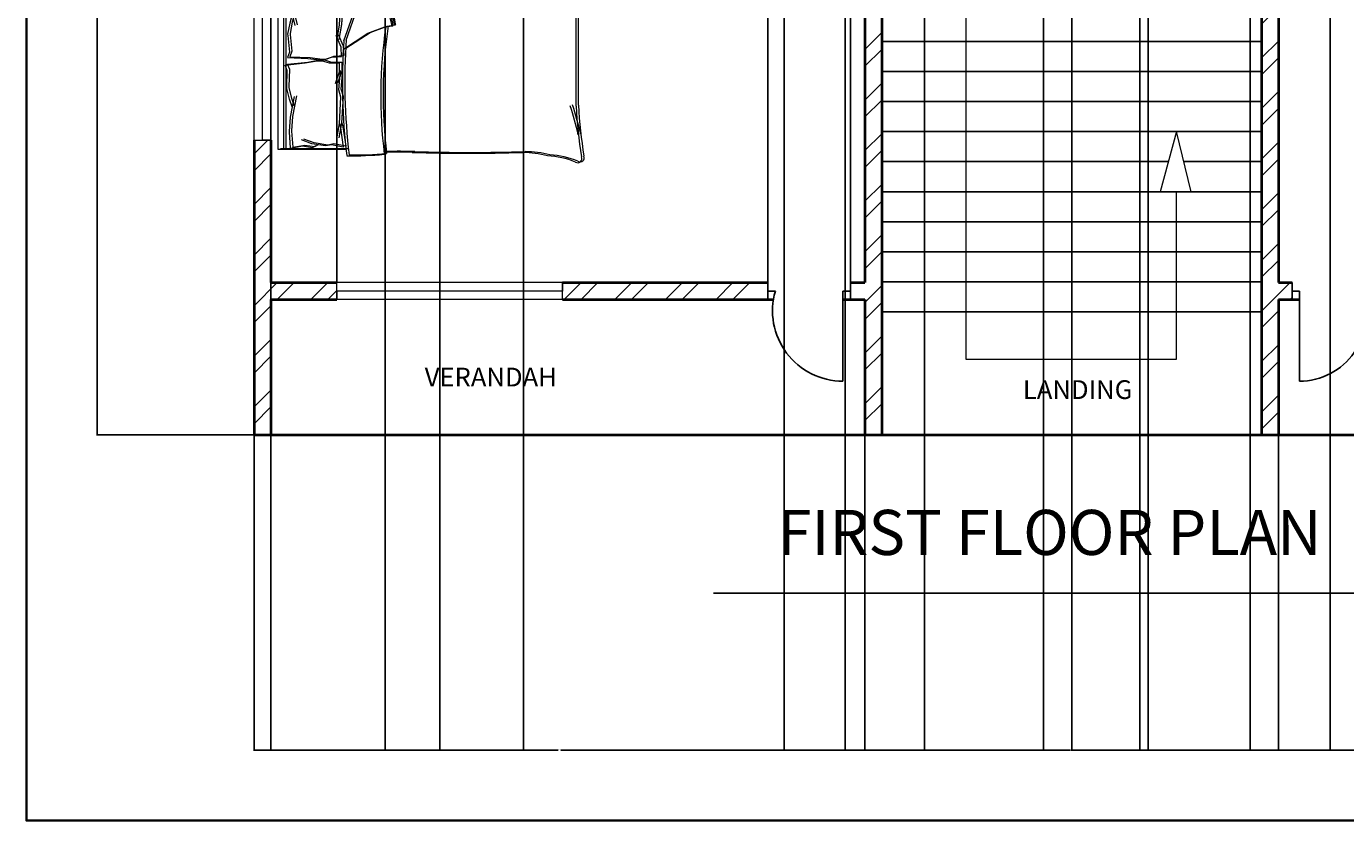
# Model space of a CAD drawing. Units: inches. Extents: x 2063 to 2617, y 1299 to 2210.
# Tile 1 of 22: x 2063 to 2414, y 1299 to 1510. Entities that reach past the tile are written whole.
import ezdxf

# ---------------------------------------------------------------- set-up
doc = ezdxf.new("R2010")
doc.units = ezdxf.units.IN
for name, color, linetype, lineweight in [('A-ANNO-DIMS', 2, 'Continuous', 18), ('A-ANNO-SYMB', 171, 'Continuous', 18), ('A-ANNO-TEXT', 7, 'Continuous', 25), ('A-ANNO-TTLB', 7, 'Continuous', 35), ('A-AREA-IDEN', 7, 'Continuous', 18), ('A-DOOR', 11, 'Continuous', 25), ('A-FLOR-STRS', 171, 'Continuous', 25), ('A-FURN', 8, 'Continuous', 18), ('A-GLAZ', 123, 'Continuous', 18), ('A-WALL', 7, 'Continuous', 40)]:
    doc.layers.add(name, color=color, linetype=linetype, lineweight=lineweight)
doc.layers.add('A-WALL-PATT', color=215, linetype='Continuous', lineweight=13, true_color=0xa953a0)
doc.styles.get("Standard").update_dxf_attribs({"font": 'arial.ttf'})
doc.dimstyles.get("Standard").update_dxf_attribs({"dimtxt": 0.18, "dimasz": 0.18, "dimexe": 0.18, "dimexo": 0.0625, "dimgap": 0.09, "dimtad": 0, "dimtih": 1, "dimtoh": 1, "dimdec": 4, "dimzin": 0, "dimdsep": 46, "dimtxsty": 'Standard', "dimcen": 0.09, "dimadec": 0, "dimazin": 0, "dimtfac": 1, "dimtdec": 4, "dimtofl": 0, "dimtmove": 0, "dimatfit": 3, "dimfxl": 1, "dimtolj": 1, "dimtzin": 0, "dimarcsym": 0})

# ---------------------------------------------------------------- blocks, each defined once
blk = doc.blocks.new('BED-DOUBLE')
for p, q in [((3.48, 63.33), (3.48, 81.44)), ((3.48, 63.33), (3.48, 81.44)), ((3.48, 81.44), (51.49, 81.44)), ((3.7, 62.69), (3.7, 80.8)), ((3.7, 62.69), (3.7, 80.8)), ((51.27, 81.44), (51.27, 54.83)), ((51.27, 81.44), (51.27, 54.83)), ((51.49, 81.44), (51.49, 80.8)), ((51.49, 80.8), (51.49, 54.19)), ((51.49, 80.8), (51.49, 54.19)), ((3.48, 79.91), (51.27, 79.91)), ((3.48, 79.91), (51.27, 79.91)), ((3.7, 79.27), (51.49, 79.27)), ((3.7, 79.27), (51.49, 79.27)), ((3.89, 78.13), (4.47, 74.95)), ((3.9, 78.11), (8.18, 78.43)), ((3.9, 78.11), (8.18, 78.43)), ((3.9, 78.13), (4.47, 74.95)), ((4.12, 77.49), (4.7, 74.31)), ((4.12, 77.49), (4.7, 74.31)), ((4.13, 77.47), (8.41, 77.8)), ((4.13, 77.47), (8.41, 77.8)), ((8.18, 78.43), (8.29, 78.42)), ((8.18, 78.43), (8.29, 78.42)), ((8.29, 78.42), (12.11, 78.13)), ((8.29, 78.42), (12.11, 78.13)), ((8.41, 77.8), (8.51, 77.78)), ((8.41, 77.8), (8.51, 77.78)), ((8.51, 77.78), (12.34, 77.49)), ((8.51, 77.78), (12.34, 77.49)), ((12.11, 78.13), (17.6, 77.12)), ((12.11, 78.13), (17.6, 77.12)), ((12.34, 77.49), (17.83, 76.48)), ((12.34, 77.49), (17.83, 76.48)), ((14.86, 77.69), (16.88, 78.42)), ((14.86, 77.69), (16.88, 78.42)), ((15.08, 77.05), (17.11, 77.78)), ((15.08, 77.05), (17.11, 77.78)), ((16.88, 78.42), (19.77, 79.14)), ((16.88, 78.42), (19.77, 79.14)), ((17.11, 77.78), (20, 78.5)), ((17.11, 77.78), (20, 78.5)), ((19.77, 79.14), (20.09, 79.14)), ((19.77, 79.14), (20.09, 79.14)), ((20, 78.5), (20.32, 78.5)), ((20, 78.5), (20.32, 78.5)), ((20.09, 79.14), (24.54, 79)), ((20.09, 79.14), (24.54, 79)), ((20.32, 78.5), (24.77, 78.36)), ((20.32, 78.5), (24.77, 78.36)), ((24.54, 79), (25.98, 79.57)), ((24.54, 79), (25.98, 79.57)), ((24.77, 78.36), (26.21, 78.93)), ((24.77, 78.36), (26.21, 78.93)), ((25.98, 79.57), (26.56, 74.22)), ((25.98, 79.57), (26.56, 74.22)), ((26.21, 78.93), (26.79, 73.58)), ((26.21, 78.93), (26.79, 73.58)), ((27.98, 78.95), (27.73, 73.58)), ((27.98, 78.95), (27.73, 73.58)), ((28.21, 78.31), (27.96, 72.94)), ((28.21, 78.31), (27.96, 72.94)), ((29.46, 78.46), (27.98, 78.95)), ((29.46, 78.46), (27.98, 78.95)), ((29.68, 77.83), (28.21, 78.31)), ((29.68, 77.83), (28.21, 78.31)), ((33.88, 78.89), (29.46, 78.46)), ((33.88, 78.89), (29.46, 78.46)), ((34.11, 78.25), (29.68, 77.83)), ((34.11, 78.25), (29.68, 77.83)), ((34.21, 78.91), (33.88, 78.89)), ((34.2, 78.91), (33.88, 78.89)), ((34.43, 78.27), (34.11, 78.25)), ((34.43, 78.27), (34.11, 78.25)), ((37.14, 78.37), (34.2, 78.91)), ((37.14, 78.37), (34.21, 78.91)), ((37.36, 77.73), (34.43, 78.27)), ((37.36, 77.73), (34.43, 78.27)), ((41.91, 78.37), (36.5, 77.02)), ((41.91, 78.37), (36.5, 77.02)), ((42.14, 77.73), (36.72, 76.38)), ((42.14, 77.73), (36.72, 76.38)), ((39.2, 77.77), (37.14, 78.37)), ((39.2, 77.77), (37.14, 78.37)), ((39.43, 77.13), (37.36, 77.73)), ((39.43, 77.13), (37.36, 77.73)), ((45.71, 78.9), (41.91, 78.37)), ((45.71, 78.9), (41.91, 78.37)), ((45.94, 78.26), (42.14, 77.73)), ((45.94, 78.26), (42.14, 77.73)), ((50.11, 78.89), (44.71, 78.98)), ((44.71, 78.98), (45.71, 78.9)), ((50.11, 78.89), (44.71, 78.98)), ((44.71, 78.98), (45.71, 78.9)), ((50.34, 78.25), (44.94, 78.34)), ((44.94, 78.34), (45.94, 78.26)), ((50.34, 78.25), (44.94, 78.34)), ((44.94, 78.34), (45.94, 78.26)), ((50.11, 78.89), (49.73, 75.68)), ((50.11, 78.89), (49.73, 75.68)), ((50.34, 78.25), (49.96, 75.04)), ((50.34, 78.25), (49.96, 75.04)), ((4.47, 74.95), (4.04, 72.34)), ((4.47, 74.95), (4.04, 72.34)), ((4.7, 74.31), (4.27, 71.7)), ((4.7, 74.31), (4.27, 71.7)), ((5.05, 72.49), (6.06, 75.24)), ((5.05, 72.49), (6.06, 75.24)), ((5.28, 71.85), (6.29, 74.6)), ((5.28, 71.85), (6.29, 74.6)), ((26.56, 74.22), (27.14, 71.04)), ((26.56, 74.22), (27.14, 71.04)), ((49.31, 73.19), (48.13, 75.87)), ((49.31, 73.19), (48.13, 75.87)), ((49.54, 72.55), (48.36, 75.23)), ((49.54, 72.55), (48.36, 75.23)), ((49.73, 75.68), (50.33, 73.11)), ((49.73, 75.68), (50.33, 73.11)), ((49.96, 75.04), (50.56, 72.47)), ((49.96, 75.04), (50.56, 72.47)), ((4.04, 72.34), (4.62, 71.33)), ((4.04, 72.34), (4.62, 71.33)), ((4.27, 71.7), (4.85, 70.69)), ((4.27, 71.7), (4.85, 70.69)), ((4.47, 68.87), (5.05, 72.49)), ((4.47, 68.87), (5.05, 72.49)), ((4.7, 68.23), (5.28, 71.85)), ((4.7, 68.23), (5.28, 71.85)), ((26.79, 73.58), (27.37, 70.4)), ((26.79, 73.58), (27.37, 70.4)), ((27.14, 71.04), (27.14, 69.74)), ((27.14, 71.04), (27.14, 69.74)), ((27.73, 73.58), (27.36, 70.37)), ((27.73, 73.58), (27.36, 70.37)), ((27.36, 70.37), (27.44, 69.07)), ((27.36, 70.37), (27.44, 69.07)), ((27.37, 70.4), (27.37, 69.1)), ((27.37, 70.4), (27.37, 69.1)), ((27.96, 72.94), (27.58, 69.73)), ((27.96, 72.94), (27.58, 69.73)), ((50.11, 69.61), (49.31, 73.19)), ((50.11, 69.61), (49.31, 73.19)), ((50.34, 68.98), (49.54, 72.55)), ((50.34, 68.98), (49.54, 72.55)), ((50.33, 73.11), (49.81, 72.06)), ((50.33, 73.11), (49.82, 72.06)), ((50.56, 72.47), (50.04, 71.42)), ((50.56, 72.47), (50.04, 71.42)), ((4.18, 64.1), (4.76, 67.28)), ((4.18, 64.1), (4.76, 67.28)), ((4.76, 67.28), (4.47, 68.87)), ((4.76, 67.28), (4.47, 68.87)), ((4.99, 66.64), (4.7, 68.23)), ((4.99, 66.64), (4.7, 68.23)), ((27.14, 69.74), (26.56, 67.86)), ((27.14, 69.74), (26.56, 67.86)), ((26.56, 67.86), (26.56, 65.18)), ((26.56, 67.86), (26.56, 65.18)), ((27.37, 69.1), (26.79, 67.22)), ((27.37, 69.1), (26.79, 67.22)), ((26.79, 67.22), (26.79, 64.54)), ((26.79, 67.22), (26.79, 64.54)), ((27.44, 69.07), (28.13, 67.23)), ((27.44, 69.07), (28.13, 67.23)), ((27.58, 69.73), (27.66, 68.43)), ((27.58, 69.73), (27.66, 68.43)), ((27.66, 68.43), (28.36, 66.59)), ((27.66, 68.43), (28.36, 66.59)), ((28.13, 67.23), (28.3, 64.55)), ((28.13, 67.23), (28.3, 64.55)), ((49.92, 68.01), (50.11, 69.61)), ((49.92, 68.01), (50.11, 69.61)), ((50.7, 64.87), (49.92, 68.01)), ((50.7, 64.87), (49.92, 68.01)), ((50.15, 67.37), (50.34, 68.98)), ((50.15, 67.37), (50.34, 68.98)), ((50.93, 64.23), (50.15, 67.37)), ((50.93, 64.23), (50.15, 67.37)), ((9.28, 64.83), (4.18, 64.1)), ((9.28, 64.83), (4.18, 64.1)), ((4.41, 63.46), (4.99, 66.64)), ((4.41, 63.46), (4.99, 66.64)), ((9.51, 64.19), (4.41, 63.46)), ((9.51, 64.19), (4.41, 63.46)), ((6.38, 65.82), (10.41, 65.15)), ((6.38, 65.82), (10.41, 65.15)), ((6.61, 65.18), (10.64, 64.51)), ((6.61, 65.18), (10.64, 64.51)), ((10.41, 65.15), (9.28, 64.83)), ((10.41, 65.15), (9.28, 64.83)), ((10.64, 64.51), (9.51, 64.19)), ((10.64, 64.51), (9.51, 64.19)), ((10.41, 65.15), (17.42, 64.72)), ((10.41, 65.15), (17.42, 64.72)), ((10.64, 64.51), (17.65, 64.08)), ((10.64, 64.51), (17.65, 64.08)), ((17.42, 64.72), (19.38, 65.27)), ((17.42, 64.72), (19.38, 65.27)), ((17.65, 64.08), (19.61, 64.64)), ((17.65, 64.08), (19.61, 64.64)), ((19.38, 65.27), (24.52, 64.87)), ((19.38, 65.27), (24.52, 64.87)), ((19.61, 64.64), (24.74, 64.23)), ((19.61, 64.64), (24.74, 64.23)), ((24.1, 65.18), (20.96, 66.27)), ((24.1, 65.18), (20.96, 66.27)), ((24.33, 64.54), (21.19, 65.63)), ((24.33, 64.54), (21.19, 65.63)), ((26.56, 65.18), (24.1, 65.18)), ((26.56, 65.18), (24.1, 65.18)), ((26.79, 64.54), (24.33, 64.54)), ((26.79, 64.54), (24.33, 64.54)), ((28.3, 64.55), (30.75, 64.7)), ((28.3, 64.55), (30.75, 64.7)), ((28.36, 66.59), (28.53, 63.91)), ((28.36, 66.59), (28.53, 63.91)), ((28.53, 63.91), (30.98, 64.06)), ((28.53, 63.91), (30.98, 64.06)), ((30.26, 64.06), (34.45, 57.57)), ((30.26, 64.06), (34.45, 57.57)), ((30.49, 63.42), (34.68, 56.93)), ((30.49, 63.42), (34.68, 56.93)), ((30.75, 64.7), (33.82, 65.99)), ((30.75, 64.7), (33.82, 65.99)), ((30.98, 64.06), (34.05, 65.35)), ((30.98, 64.06), (34.05, 65.35)), ((40.64, 61.13), (32.31, 64.06)), ((40.64, 61.13), (32.31, 64.06)), ((40.87, 60.49), (32.53, 63.42)), ((40.87, 60.49), (32.54, 63.42)), ((32.56, 65.82), (36.6, 65.15)), ((32.56, 65.82), (36.6, 65.15)), ((32.79, 65.18), (36.83, 64.51)), ((32.79, 65.18), (36.82, 64.51)), ((36.6, 65.15), (43.61, 64.72)), ((36.6, 65.15), (43.61, 64.72)), ((36.82, 64.51), (43.83, 64.08)), ((36.83, 64.51), (43.84, 64.08)), ((43.61, 64.72), (45.57, 65.27)), ((43.61, 64.72), (45.57, 65.27)), ((43.83, 64.08), (45.8, 64.64)), ((43.84, 64.08), (45.8, 64.64)), ((45.57, 65.27), (50.7, 64.87)), ((45.57, 65.27), (50.7, 64.87)), ((45.8, 64.64), (50.93, 64.23)), ((45.8, 64.64), (50.93, 64.23)), ((46.22, 59.11), (40.64, 61.13)), ((46.22, 59.11), (40.64, 61.13)), ((46.45, 58.48), (40.87, 60.49)), ((46.45, 58.48), (40.87, 60.49)), ((34.45, 57.57), (36.15, 53.08)), ((34.45, 57.57), (36.15, 53.08)), ((34.68, 56.93), (36.38, 52.44)), ((34.68, 56.93), (36.38, 52.44)), ((49.16, 56.95), (46.22, 59.11)), ((49.16, 56.95), (46.22, 59.11)), ((49.39, 56.31), (46.45, 58.48)), ((49.39, 56.31), (46.45, 58.48)), ((52.87, 53.7), (49.16, 56.95)), ((52.87, 53.7), (49.16, 56.95)), ((53.1, 53.06), (49.39, 56.31)), ((53.1, 53.06), (49.39, 56.31)), ((36.15, 53.08), (36.46, 51.07)), ((36.15, 53.08), (36.46, 51.07)), ((40.95, 52.61), (44.36, 53.08)), ((40.95, 52.61), (44.36, 53.08)), ((44.36, 53.08), (48.23, 53.39)), ((44.36, 53.08), (48.23, 53.39)), ((44.59, 52.44), (48.46, 52.75)), ((44.59, 52.44), (48.46, 52.75)), ((48.23, 53.39), (51.33, 53.08)), ((48.23, 53.39), (51.33, 53.08)), ((48.46, 52.75), (51.56, 52.44)), ((48.46, 52.75), (51.56, 52.44)), ((51.33, 53.08), (52.87, 53.7)), ((51.33, 53.08), (52.87, 53.7)), ((51.56, 52.44), (53.1, 53.06)), ((51.56, 52.44), (53.1, 53.06)), ((52.95, 51.95), (52.87, 53.7, 3.87)), ((52.95, 51.95), (52.87, 53.7, 3.87)), ((53.18, 51.31), (53.1, 53.06, 3.87)), ((53.18, 51.31), (53.1, 53.06, 3.87)), ((36.38, 52.44), (36.69, 50.43)), ((36.38, 52.44), (36.69, 50.43)), ((36.46, 51.07), (38.94, 51.69)), ((36.46, 51.07), (38.94, 51.69)), ((36.69, 50.43), (39.17, 51.05)), ((36.69, 50.43), (39.17, 51.05)), ((38.94, 51.69), (40.95, 52.61)), ((38.94, 51.69), (40.95, 52.61)), ((39.17, 51.05), (41.18, 51.97)), ((39.17, 51.05), (41.18, 51.97)), ((41.18, 51.97), (44.59, 52.44)), ((41.18, 51.97), (44.59, 52.44)), ((15.06, 2.2), (39.68, 2.2)), ((15.06, 2.2), (39.68, 2.2)), ((15.29, 1.56), (39.91, 1.56)), ((15.29, 1.56), (39.91, 1.56))]:
    blk.add_line(p, q)
for centre, radius, start, end in [((85.16, 61.35), 83.31, 178.7218, 185.604), ((85.16, 61.35), 83.31, 178.7218, 185.604), ((21.36, -100.61), 164.97, 86.0865, 96.7821), ((21.36, -100.61), 164.97, 86.0865, 96.7821), ((21.59, -101.25), 164.97, 86.0865, 96.7821), ((21.59, -101.25), 164.97, 86.0865, 96.7821), ((85.39, 60.71), 83.31, 178.7218, 185.604), ((85.39, 60.71), 83.31, 178.7218, 185.604), ((17.76, -74.87), 129.02, 81.7845, 96.9006), ((17.76, -74.87), 129.02, 81.7845, 96.9006), ((17.98, -75.51), 129.02, 81.7845, 96.9006), ((17.98, -75.51), 129.02, 81.7845, 96.9006), ((-167.31, 50.27), 170.11, 358.4762, 1.0082), ((-167.31, 50.27), 170.11, 358.4762, 1.0082), ((-167.08, 49.63), 170.11, 358.4762, 1.0082), ((-167.08, 49.63), 170.11, 358.4762, 1.0082), ((36.64, 51), 0.185, 160.2464, 271.1377), ((36.64, 51), 0.185, 160.2464, 271.1377), ((31.15, 79.96), 29.65, 280.6617, 289.8806), ((31.15, 79.96), 29.65, 280.6617, 289.8806), ((36.87, 50.36), 0.185, 160.2464, 271.1377), ((36.86, 50.36), 0.185, 160.2464, 271.1377), ((31.38, 79.32), 29.65, 280.6617, 289.8806), ((31.38, 79.32), 29.65, 280.6617, 289.8806), ((43.74, 46.38), 6.22, 78.6608, 113.7384), ((43.74, 46.38), 6.22, 78.6608, 113.7384), ((43.97, 45.74), 6.22, 78.6608, 113.7384), ((43.97, 45.74), 6.22, 78.6608, 113.7384), ((51.33, 88.1), 36.18, 259.8763, 272.5657), ((51.33, 88.1), 36.18, 259.8763, 272.5657), ((51.56, 87.46), 36.18, 259.8763, 272.5657), ((51.56, 87.46), 36.18, 259.8763, 272.5657), ((182.27, 45.13), 129.5, 176.9791, 183.8365), ((182.27, 45.13), 129.5, 176.9791, 183.8365), ((182.49, 44.49), 129.5, 176.9791, 183.8365), ((182.49, 44.49), 129.5, 176.9791, 183.8365), ((484.82, 30.83), 482.31, 178.2277, 181.7185), ((484.82, 30.83), 482.31, 178.2277, 181.7185), ((485.05, 30.19), 482.31, 178.2277, 181.7185), ((485.05, 30.19), 482.31, 178.2277, 181.7185), ((-4508.74, 13.62), 4561.86, 0.00217, 0.28689), ((-4508.74, 13.62), 4561.86, 0.00217, 0.28689), ((-4508.51, 12.98), 4561.86, 0.00217, 0.28689), ((-4508.51, 12.98), 4561.86, 0.00217, 0.28689), ((-26.9, 16.93), 29.63, 346.0648, 358.9113), ((-26.9, 16.93), 29.63, 346.0648, 358.9113), ((-26.67, 16.29), 29.63, 346.0648, 358.9113), ((-26.67, 16.29), 29.63, 346.0648, 358.9113), ((76.16, 12.78), 23.07, 177.4714, 206.4681), ((76.16, 12.78), 23.07, 177.4714, 206.4681), ((76.39, 12.14), 23.07, 177.4714, 206.4681), ((76.39, 12.14), 23.07, 177.4714, 206.4681), ((-21.66, 11.17), 23.56, 337.9751, 356.652), ((-21.66, 11.17), 23.56, 337.9751, 356.652), ((-21.43, 10.53), 23.56, 337.9751, 356.652), ((-21.43, 10.53), 23.56, 337.9751, 356.652), ((-17.22, 105.16), 106.46, 283.3832, 287.7053), ((-17.22, 105.16), 106.46, 283.3832, 287.7053), ((1.09, 1.73), 1.09, 146.1736, 293.4781), ((1.09, 1.73), 1.09, 146.1736, 293.4781), ((1.32, 1.09), 1.09, 146.1736, 293.4781), ((1.32, 1.09), 1.09, 146.1736, 293.4781), ((21.43, -119.39), 121.76, 92.9958, 99.4091), ((21.43, -119.39), 121.76, 92.9958, 99.4091), ((21.66, -120.03), 121.76, 92.9958, 99.4091), ((21.66, -120.03), 121.76, 92.9958, 99.4091), ((-16.99, 104.52), 106.46, 283.3832, 287.7053), ((-16.99, 104.52), 106.46, 283.3832, 287.7053), ((41.15, -130.83), 133.04, 84.4998, 90.6351), ((41.15, -130.83), 133.04, 84.4998, 90.6351), ((41.38, -131.47), 133.04, 84.4998, 90.6351), ((41.38, -131.47), 133.04, 84.4998, 90.6351), ((54.41, 2.57), 1.1, 242.6588, 356.02), ((54.41, 2.57), 1.1, 242.6588, 356.02), ((54.64, 1.93), 1.1, 242.6588, 356.02), ((54.64, 1.93), 1.1, 242.6588, 356.02)]:
    blk.add_arc(centre, radius, start, end)
blk = doc.blocks.new('WIN-60IN')
for p, q in [((0, 60), (4.5, 60)), ((0, 60), (0, 0)), ((4.5, 60), (2.25, 60)), ((2.25, 60), (2.25, 0)), ((4.5, 60), (4.5, 0)), ((2.25, 0), (0, 0)), ((0, 0), (4.5, 0))]:
    blk.add_line(p, q)
blk = doc.blocks.new('*D32')
at = {"layer": 'A-ANNO-DIMS', "color": 0, "lineweight": -2, "transparency": 16777216}
for p, q in [((2123.08, 2128.81), (2081.21, 2128.81)), ((2081.39, 2128.63), (2081.39, 1765.49)), ((2081.39, 1401.99), (2081.39, 1765.13)), ((2123.08, 1401.81), (2081.21, 1401.81))]:
    blk.add_line(p, q, dxfattribs=at)
at = {"layer": 'A-ANNO-DIMS', "color": 0, "transparency": 16777216}
for points in [[(2081.36, 2128.63), (2081.42, 2128.63), (2081.39, 2128.81)], [(2081.36, 1401.99), (2081.42, 1401.99), (2081.39, 1401.81)]]:
    blk.add_solid(points, dxfattribs=at)
at = {"layer": 'Defpoints', "color": 0, "transparency": 16777216}
for p in [(2081.39, 2128.81), (2123.14, 2128.81), (2123.14, 1401.81)]:
    blk.add_point(p, dxfattribs=at)
at = {"layer": 'A-ANNO-DIMS', "color": 0, "transparency": 16777216, "insert": (2081.39, 1765.31), "char_height": 0.18, "attachment_point": 5}
blk.add_mtext('\\A1;727', dxfattribs=at)
blk = doc.blocks.new('*D33')
at = {"layer": 'A-ANNO-DIMS', "color": 0, "lineweight": -2, "transparency": 16777216}
for p, q in [((2123.14, 1401.75), (2123.14, 1317.7)), ((2285.64, 1401.75), (2285.64, 1317.7)), ((2123.32, 1317.88), (2204.01, 1317.88)), ((2285.46, 1317.88), (2204.78, 1317.88))]:
    blk.add_line(p, q, dxfattribs=at)
at = {"layer": 'A-ANNO-DIMS', "color": 0, "transparency": 16777216}
for points in [[(2123.32, 1317.91), (2123.32, 1317.85), (2123.14, 1317.88)], [(2285.46, 1317.91), (2285.46, 1317.85), (2285.64, 1317.88)]]:
    blk.add_solid(points, dxfattribs=at)
at = {"layer": 'Defpoints', "color": 0, "transparency": 16777216}
for p in [(2123.14, 1401.81), (2285.64, 1401.81), (2285.64, 1317.88)]:
    blk.add_point(p, dxfattribs=at)
at = {"layer": 'A-ANNO-DIMS', "color": 0, "transparency": 16777216, "insert": (2204.39, 1317.88), "char_height": 0.18, "attachment_point": 5}
blk.add_mtext('\\A1;162.5', dxfattribs=at)
blk = doc.blocks.new('*D34')
at = {"layer": 'A-ANNO-DIMS', "color": 0, "lineweight": -2, "transparency": 16777216}
for p, q in [((2285.64, 1401.75), (2285.64, 1317.7)), ((2395.64, 1401.75), (2395.64, 1317.7)), ((2285.82, 1317.88), (2340.36, 1317.88)), ((2395.46, 1317.88), (2340.92, 1317.88))]:
    blk.add_line(p, q, dxfattribs=at)
at = {"layer": 'A-ANNO-DIMS', "color": 0, "transparency": 16777216}
for points in [[(2285.82, 1317.91), (2285.82, 1317.85), (2285.64, 1317.88)], [(2395.46, 1317.91), (2395.46, 1317.85), (2395.64, 1317.88)]]:
    blk.add_solid(points, dxfattribs=at)
at = {"layer": 'Defpoints', "color": 0, "transparency": 16777216}
for p in [(2285.64, 1401.81), (2395.64, 1401.81), (2395.64, 1317.88)]:
    blk.add_point(p, dxfattribs=at)
at = {"layer": 'A-ANNO-DIMS', "color": 0, "transparency": 16777216, "insert": (2340.64, 1317.88), "char_height": 0.18, "attachment_point": 5}
blk.add_mtext('\\A1;110', dxfattribs=at)
blk = doc.blocks.new('*D35')
at = {"layer": 'A-ANNO-DIMS', "color": 0, "lineweight": -2, "transparency": 16777216}
for p, q in [((2395.64, 1401.75), (2395.64, 1317.7)), ((2553.64, 1401.75), (2553.64, 1317.7)), ((2395.82, 1317.88), (2474.36, 1317.88)), ((2553.46, 1317.88), (2474.92, 1317.88))]:
    blk.add_line(p, q, dxfattribs=at)
at = {"layer": 'A-ANNO-DIMS', "color": 0, "transparency": 16777216}
for points in [[(2395.82, 1317.91), (2395.82, 1317.85), (2395.64, 1317.88)], [(2553.46, 1317.91), (2553.46, 1317.85), (2553.64, 1317.88)]]:
    blk.add_solid(points, dxfattribs=at)
at = {"layer": 'Defpoints', "color": 0, "transparency": 16777216}
for p in [(2395.64, 1401.81), (2553.64, 1401.81), (2553.64, 1317.88)]:
    blk.add_point(p, dxfattribs=at)
at = {"layer": 'A-ANNO-DIMS', "color": 0, "transparency": 16777216, "insert": (2474.64, 1317.88), "char_height": 0.18, "attachment_point": 5}
blk.add_mtext('\\A1;158', dxfattribs=at)
blk = doc.blocks.new('*D49')
at = {"layer": 'A-ANNO-DIMS', "color": 0, "lineweight": -2, "transparency": 16777216}
for p, q in [((2127.64, 2124.25), (2127.64, 1317.7)), ((2158.04, 2124.25), (2158.04, 1317.7)), ((2127.82, 1317.88), (2142.38, 1317.88)), ((2157.86, 1317.88), (2143.31, 1317.88))]:
    blk.add_line(p, q, dxfattribs=at)
at = {"layer": 'A-ANNO-DIMS', "color": 0, "transparency": 16777216}
for points in [[(2127.82, 1317.91), (2127.82, 1317.85), (2127.64, 1317.88)], [(2157.86, 1317.91), (2157.86, 1317.85), (2158.04, 1317.88)]]:
    blk.add_solid(points, dxfattribs=at)
at = {"layer": 'Defpoints', "color": 0, "transparency": 16777216}
for p in [(2127.64, 2124.31), (2158.04, 2124.31), (2158.04, 1317.88)]:
    blk.add_point(p, dxfattribs=at)
at = {"layer": 'A-ANNO-DIMS', "color": 0, "transparency": 16777216, "insert": (2142.84, 1317.88), "char_height": 0.18, "attachment_point": 5}
blk.add_mtext('\\A1;30.396', dxfattribs=at)
blk = doc.blocks.new('*D50')
at = {"layer": 'A-ANNO-DIMS', "color": 0, "lineweight": -2, "transparency": 16777216}
for p, q in [((2264.14, 2124.25), (2264.14, 1317.7)), ((2280.35, 2124.25), (2280.35, 1317.7)), ((2264.32, 1317.88), (2271.79, 1317.88)), ((2280.17, 1317.88), (2272.7, 1317.88))]:
    blk.add_line(p, q, dxfattribs=at)
at = {"layer": 'A-ANNO-DIMS', "color": 0, "transparency": 16777216}
for points in [[(2264.32, 1317.91), (2264.32, 1317.85), (2264.14, 1317.88)], [(2280.17, 1317.91), (2280.17, 1317.85), (2280.35, 1317.88)]]:
    blk.add_solid(points, dxfattribs=at)
at = {"layer": 'Defpoints', "color": 0, "transparency": 16777216}
for p in [(2264.14, 2124.31), (2280.35, 2124.31), (2280.35, 1317.88)]:
    blk.add_point(p, dxfattribs=at)
at = {"layer": 'A-ANNO-DIMS', "color": 0, "transparency": 16777216, "insert": (2272.25, 1317.88), "char_height": 0.18, "attachment_point": 5}
blk.add_mtext('\\A1;16.204', dxfattribs=at)
blk = doc.blocks.new('*D51')
at = {"layer": 'A-ANNO-DIMS', "color": 0, "lineweight": -2, "transparency": 16777216}
for p, q in [((2340.64, 2124.25), (2340.64, 1317.7)), ((2358.75, 2124.25), (2358.75, 1317.7)), ((2340.82, 1317.88), (2349.24, 1317.88)), ((2358.57, 1317.88), (2350.15, 1317.88))]:
    blk.add_line(p, q, dxfattribs=at)
at = {"layer": 'A-ANNO-DIMS', "color": 0, "transparency": 16777216}
for points in [[(2340.82, 1317.91), (2340.82, 1317.85), (2340.64, 1317.88)], [(2358.57, 1317.91), (2358.57, 1317.85), (2358.75, 1317.88)]]:
    blk.add_solid(points, dxfattribs=at)
at = {"layer": 'Defpoints', "color": 0, "transparency": 16777216}
for p in [(2340.64, 2124.31), (2358.75, 2124.31), (2358.75, 1317.88)]:
    blk.add_point(p, dxfattribs=at)
at = {"layer": 'A-ANNO-DIMS', "color": 0, "transparency": 16777216, "insert": (2349.7, 1317.88), "char_height": 0.18, "attachment_point": 5}
blk.add_mtext('\\A1;18.106', dxfattribs=at)
blk = doc.blocks.new('*D54')
at = {"layer": 'A-ANNO-DIMS', "color": 0, "lineweight": -2, "transparency": 16777216}
for p, q in [((2340.64, 2124.25), (2340.64, 1317.7)), ((2360.96, 2104.46), (2360.96, 1317.7)), ((2340.82, 1317.88), (2350.34, 1317.88)), ((2360.78, 1317.88), (2351.27, 1317.88))]:
    blk.add_line(p, q, dxfattribs=at)
at = {"layer": 'A-ANNO-DIMS', "color": 0, "transparency": 16777216}
for points in [[(2340.82, 1317.91), (2340.82, 1317.85), (2340.64, 1317.88)], [(2360.78, 1317.91), (2360.78, 1317.85), (2360.96, 1317.88)]]:
    blk.add_solid(points, dxfattribs=at)
at = {"layer": 'Defpoints', "color": 0, "transparency": 16777216}
for p in [(2340.64, 2124.31), (2360.96, 2104.52), (2360.96, 1317.88)]:
    blk.add_point(p, dxfattribs=at)
at = {"layer": 'A-ANNO-DIMS', "color": 0, "transparency": 16777216, "insert": (2350.8, 1317.88), "char_height": 0.18, "attachment_point": 5}
blk.add_mtext('\\A1;20.317', dxfattribs=at)
blk = doc.blocks.new('*D55')
at = {"layer": 'A-ANNO-DIMS', "color": 0, "lineweight": -2, "transparency": 16777216}
for p, q in [((2388.15, 1975.75), (2388.15, 1317.7)), ((2409.37, 1975.75), (2409.37, 1317.7)), ((2388.33, 1317.88), (2398.3, 1317.88)), ((2409.19, 1317.88), (2399.23, 1317.88))]:
    blk.add_line(p, q, dxfattribs=at)
at = {"layer": 'A-ANNO-DIMS', "color": 0, "transparency": 16777216}
for points in [[(2388.33, 1317.91), (2388.33, 1317.85), (2388.15, 1317.88)], [(2409.19, 1317.91), (2409.19, 1317.85), (2409.37, 1317.88)]]:
    blk.add_solid(points, dxfattribs=at)
at = {"layer": 'Defpoints', "color": 0, "transparency": 16777216}
for p in [(2388.15, 1975.81), (2409.37, 1975.81), (2409.37, 1317.88)]:
    blk.add_point(p, dxfattribs=at)
at = {"layer": 'A-ANNO-DIMS', "color": 0, "transparency": 16777216, "insert": (2398.76, 1317.88), "char_height": 0.18, "attachment_point": 5}
blk.add_mtext('\\A1;21.225', dxfattribs=at)
blk = doc.blocks.new('*D57')
at = {"layer": 'A-ANNO-DIMS', "color": 0, "lineweight": -2, "transparency": 16777216}
for p, q in [((2172.52, 1868.25), (2172.52, 1317.7)), ((2194.82, 1868.25), (2194.82, 1317.7)), ((2172.7, 1317.88), (2183.2, 1317.88)), ((2194.64, 1317.88), (2184.14, 1317.88))]:
    blk.add_line(p, q, dxfattribs=at)
at = {"layer": 'A-ANNO-DIMS', "color": 0, "transparency": 16777216}
for points in [[(2172.7, 1317.91), (2172.7, 1317.85), (2172.52, 1317.88)], [(2194.64, 1317.91), (2194.64, 1317.85), (2194.82, 1317.88)]]:
    blk.add_solid(points, dxfattribs=at)
at = {"layer": 'Defpoints', "color": 0, "transparency": 16777216}
for p in [(2172.52, 1868.31), (2194.82, 1868.31), (2194.82, 1317.88)]:
    blk.add_point(p, dxfattribs=at)
at = {"layer": 'A-ANNO-DIMS', "color": 0, "transparency": 16777216, "insert": (2183.67, 1317.88), "char_height": 0.18, "attachment_point": 5}
blk.add_mtext('\\A1;22.305', dxfattribs=at)
blk = doc.blocks.new('*D60')
at = {"layer": 'A-ANNO-DIMS', "color": 0, "lineweight": -2, "transparency": 16777216}
for p, q in [((2301.46, 1614.75), (2301.46, 1317.7)), ((2333.14, 1614.75), (2333.14, 1317.7)), ((2301.64, 1317.88), (2316.84, 1317.88)), ((2332.96, 1317.88), (2317.76, 1317.88))]:
    blk.add_line(p, q, dxfattribs=at)
at = {"layer": 'A-ANNO-DIMS', "color": 0, "transparency": 16777216}
for points in [[(2301.64, 1317.91), (2301.64, 1317.85), (2301.46, 1317.88)], [(2332.96, 1317.91), (2332.96, 1317.85), (2333.14, 1317.88)]]:
    blk.add_solid(points, dxfattribs=at)
at = {"layer": 'Defpoints', "color": 0, "transparency": 16777216}
for p in [(2301.46, 1614.81), (2333.14, 1614.81), (2333.14, 1317.88)]:
    blk.add_point(p, dxfattribs=at)
at = {"layer": 'A-ANNO-DIMS', "color": 0, "transparency": 16777216, "insert": (2317.3, 1317.88), "char_height": 0.18, "attachment_point": 5}
blk.add_mtext('\\A1;31.684', dxfattribs=at)
blk = doc.blocks.new('*D61')
at = {"layer": 'A-ANNO-DIMS', "color": 0, "lineweight": -2, "transparency": 16777216}
for p, q in [((2127.64, 1442.37), (2127.64, 2170.74)), ((2127.82, 2170.56), (2136.03, 2170.56)), ((2144.97, 2170.56), (2136.77, 2170.56)), ((2145.15, 1442.37), (2145.15, 2170.74))]:
    blk.add_line(p, q, dxfattribs=at)
at = {"layer": 'A-ANNO-DIMS', "color": 0, "transparency": 16777216}
for points in [[(2127.82, 2170.59), (2127.82, 2170.53), (2127.64, 2170.56)], [(2144.97, 2170.59), (2144.97, 2170.53), (2145.15, 2170.56)]]:
    blk.add_solid(points, dxfattribs=at)
at = {"layer": 'Defpoints', "color": 0, "transparency": 16777216}
for p in [(2145.15, 2170.56), (2127.64, 1442.31), (2145.15, 1442.31)]:
    blk.add_point(p, dxfattribs=at)
at = {"layer": 'A-ANNO-DIMS', "color": 0, "transparency": 16777216, "insert": (2136.4, 2170.56), "char_height": 0.18, "attachment_point": 5}
blk.add_mtext('\\A1;17.51', dxfattribs=at)
blk = doc.blocks.new('*D62')
at = {"layer": 'A-ANNO-DIMS', "color": 0, "lineweight": -2, "transparency": 16777216}
for p, q in [((2259.81, 1437.87), (2259.81, 2170.74)), ((2259.99, 2170.56), (2270.4, 2170.56)), ((2281.61, 2170.56), (2271.19, 2170.56)), ((2281.79, 1437.87), (2281.79, 2170.74))]:
    blk.add_line(p, q, dxfattribs=at)
at = {"layer": 'A-ANNO-DIMS', "color": 0, "transparency": 16777216}
for points in [[(2259.99, 2170.59), (2259.99, 2170.53), (2259.81, 2170.56)], [(2281.61, 2170.59), (2281.61, 2170.53), (2281.79, 2170.56)]]:
    blk.add_solid(points, dxfattribs=at)
at = {"layer": 'Defpoints', "color": 0, "transparency": 16777216}
for p in [(2281.79, 2170.56), (2259.81, 1437.81), (2281.79, 1437.81)]:
    blk.add_point(p, dxfattribs=at)
at = {"layer": 'A-ANNO-DIMS', "color": 0, "transparency": 16777216, "insert": (2270.8, 2170.56), "char_height": 0.18, "attachment_point": 5}
blk.add_mtext('\\A1;21.98', dxfattribs=at)

msp = doc.modelspace()

# ---------------------------------------------------------------- hatches: boundary and pattern name
at = {"layer": 'A-WALL-PATT'}
h = msp.add_hatch(dxfattribs=at)
h.set_pattern_fill('ANSI32', color=256)
h.paths.add_polyline_path([(2553.6442, 2128.8122), (2511.1703, 2128.8122), (2511.1703, 2124.3122), (2549.1442, 2124.3122), (2549.1442, 2095.662), (2553.6442, 2095.662)])
h.paths.add_polyline_path([(2553.6442, 2035.662), (2549.1442, 2035.662), (2549.1442, 1980.3122), (2503.7214, 1980.3122), (2503.7214, 1975.8122), (2549.1442, 1975.8122), (2549.1442, 1962.9693), (2553.6442, 1962.9693)])
h.paths.add_polyline_path([(2553.6442, 1938.9693), (2549.1442, 1938.9693), (2549.1442, 1927.8122), (2477.1442, 1927.8122), (2477.1442, 1975.8122), (2481.2918, 1975.8122), (2481.2918, 1980.3122), (2453.2648, 1980.3122), (2453.2648, 1975.8122), (2472.6442, 1975.8122), (2472.6442, 1868.3122), (2400.6442, 1868.3122), (2400.6442, 1861.3782), (2405.1442, 1861.3782), (2405.1442, 1863.8122), (2480.9699, 1863.8122), (2480.9699, 1866.0622), (2480.9699, 1868.3122), (2477.1442, 1868.3122), (2477.1442, 1923.3122), (2549.1442, 1923.3122), (2549.1442, 1908.8504), (2553.6442, 1908.8504)])
h.paths.add_polyline_path([(2553.6442, 1884.8504), (2549.1442, 1884.8504), (2549.1442, 1868.3122), (2501.0636, 1868.3122), (2501.0636, 1863.8122), (2549.1442, 1863.8122), (2549.1442, 1826.0298), (2553.6442, 1826.0298)])
h.paths.add_polyline_path([(2388.1504, 1980.3122), (2340.6442, 1980.3122), (2340.6442, 2124.3122), (2358.7501, 2124.3122), (2358.7501, 2128.8122), (2316.3482, 2128.8122), (2316.3482, 2124.3122), (2336.1442, 2124.3122), (2336.1442, 1980.3122), (2289.1737, 1980.3122), (2289.1737, 1975.8122), (2336.1442, 1975.8122), (2336.1442, 1619.3122), (2333.1433, 1619.3122), (2333.1433, 1614.8122), (2344.1671, 1614.8122), (2344.1671, 1617.0622), (2344.1671, 1619.3122), (2340.6442, 1619.3122), (2340.6442, 1975.8122), (2388.1504, 1975.8122), (2388.1504, 1978.0622)])
h.paths.add_polyline_path([(2290.1442, 1614.8122), (2301.4594, 1614.8122), (2301.4594, 1617.0622), (2301.4594, 1619.3122), (2285.6442, 1619.3122), (2285.6442, 1566.8122), (2280.8619, 1566.8122), (2280.8619, 1564.5622), (2280.8619, 1562.3122), (2285.6442, 1562.3122), (2285.6442, 1442.3122), (2281.7879, 1442.3122), (2281.7879, 1437.8122), (2285.6442, 1437.8122), (2285.6442, 1401.8122), (2290.1442, 1401.8122)])
h.paths.add_polyline_path([(2549.1442, 1731.8122), (2405.1442, 1731.8122), (2405.1442, 1834.4638), (2402.8942, 1834.4638), (2400.6442, 1834.4638), (2400.6442, 1727.3122), (2549.1442, 1727.3122)])
h.paths.add_polyline_path([(2553.6442, 1766.0298), (2551.3942, 1766.0298), (2549.1442, 1766.0298), (2549.1442, 1686.7767), (2553.6442, 1686.7767)])
h.paths.add_polyline_path([(2553.6442, 1638.7767), (2551.3942, 1638.7767), (2549.1442, 1638.7767), (2549.1442, 1619.3122), (2448.6442, 1619.3122), (2448.6442, 1610.5671), (2450.8942, 1610.5671), (2453.1442, 1610.5671), (2453.1442, 1614.8122), (2549.1442, 1614.8122), (2549.1442, 1601.6421), (2553.6442, 1601.6421)])
h.paths.add_polyline_path([(2553.6442, 1577.6421), (2551.3942, 1577.6421), (2549.1442, 1577.6421), (2549.1442, 1566.8122), (2453.1442, 1566.8122), (2453.1442, 1591.5045), (2451.0335, 1591.5045), (2448.6442, 1591.5045), (2448.6442, 1566.8122), (2434.0475, 1566.8122), (2434.0475, 1562.3122), (2549.1442, 1562.3122), (2549.1442, 1533.48), (2553.6442, 1533.48)])
h.paths.add_polyline_path([(2553.6442, 1473.48), (2549.1442, 1473.48), (2549.1442, 1442.3122), (2502.6258, 1442.3122), (2502.6258, 1437.8122), (2549.1442, 1437.8122), (2549.1442, 1401.8122), (2553.6442, 1401.8122)])
h.paths.add_polyline_path([(2395.6442, 1562.3122), (2400.0901, 1562.3122), (2400.0901, 1564.5622), (2400.0901, 1566.8122), (2395.6442, 1566.8122), (2395.6442, 1619.3122), (2379.1127, 1619.3122), (2379.1127, 1614.8122), (2391.1442, 1614.8122), (2391.1442, 1401.8122), (2395.6442, 1401.8122), (2395.6442, 1437.8122), (2399.2425, 1437.8122), (2399.2425, 1440.0622), (2399.2425, 1442.3122), (2395.6442, 1442.3122)])
h.paths.add_polyline_path([(2442.6258, 1442.3122), (2419.6262, 1442.3122), (2419.6262, 1437.8122), (2442.6258, 1437.8122), (2442.6258, 1440.0622)])
h.paths.add_polyline_path([(2127.6442, 1480.2532), (2125.3942, 1480.2532), (2123.1442, 1480.2532), (2123.1442, 1401.8122), (2127.6442, 1401.8122), (2127.6442, 1437.8122), (2145.1538, 1437.8122), (2145.1538, 1440.0622), (2145.1538, 1442.3122), (2127.6442, 1442.3122)])
h.paths.add_polyline_path([(2259.809, 1442.3122), (2205.1538, 1442.3122), (2205.1538, 1437.8122), (2259.809, 1437.8122), (2259.809, 1440.0622)])
h.paths.add_polyline_path([(2127.6442, 1659.7652), (2123.1442, 1659.7652), (2123.1442, 1605.5161), (2125.3942, 1605.5161), (2127.6442, 1605.5161), (2127.6442, 1614.8122), (2223.6442, 1614.8122), (2223.6442, 1611.2723), (2228.1442, 1611.2723), (2228.1442, 1619.3122), (2127.6442, 1619.3122)])
h.paths.add_polyline_path([(2244.8673, 1566.8122), (2228.1442, 1566.8122), (2228.1442, 1590.8122), (2225.8942, 1590.8122), (2223.6442, 1590.8122), (2223.6442, 1566.8122), (2127.6442, 1566.8122), (2127.6442, 1581.5161), (2123.1442, 1581.5161), (2123.1442, 1540.2532), (2127.6442, 1540.2532), (2127.6442, 1562.3122), (2244.8673, 1562.3122), (2244.8673, 1564.5622)])
h.paths.add_polyline_path([(2172.5174, 1868.3122), (2127.6442, 1868.3122), (2127.6442, 1886.5833), (2123.1442, 1886.5833), (2123.1442, 1832.6633), (2127.6442, 1832.6633), (2127.6442, 1863.8122), (2172.5174, 1863.8122), (2172.5174, 1866.0622)])
h.paths.add_polyline_path([(2276.1442, 1868.3122), (2204.1442, 1868.3122), (2204.1442, 1923.3122), (2204.1442, 1975.8122), (2224.8362, 1975.8122), (2224.8362, 1978.1097), (2224.8362, 1980.3122), (2195.0729, 1980.3122), (2195.0729, 1978.0622), (2195.0729, 1975.8122), (2199.6442, 1975.8122), (2199.6442, 1927.8122), (2127.6442, 1927.8122), (2127.6442, 1942.3492), (2123.1442, 1942.3492), (2123.1442, 1910.5833), (2127.6442, 1910.5833), (2127.6442, 1923.3122), (2199.6442, 1923.3122), (2199.6442, 1868.3122), (2194.8228, 1868.3122), (2194.8228, 1864.7337), (2194.8228, 1863.8122), (2271.6442, 1863.8122), (2271.6442, 1860.0507), (2276.1442, 1860.0507)])
h.paths.add_polyline_path([(2276.1442, 1829.994), (2273.8942, 1829.994), (2271.6442, 1829.994), (2271.6442, 1731.8122), (2127.6442, 1731.8122), (2127.6442, 1772.6633), (2123.1442, 1772.6633), (2123.1442, 1707.7652), (2127.6442, 1707.7652), (2127.6442, 1727.3122), (2276.1442, 1727.3122)])
h.paths.add_polyline_path([(2127.6442, 2022.1152), (2123.1442, 2022.1152), (2123.1442, 1966.3492), (2127.6442, 1966.3492), (2127.6442, 1975.8122), (2174.2082, 1975.8122), (2174.2082, 1978.0622), (2174.2082, 1980.3122), (2127.6442, 1980.3122)])
h.paths.add_polyline_path([(2361.9755, 1678.588), (2398.4558, 1678.588), (2398.4558, 1697.2453), (2361.9755, 1697.2453)], flags=9)
h.paths.add_polyline_path([(2351.5397, 1780.4072), (2386.1987, 1780.4072), (2386.1987, 1790.7107), (2351.5397, 1790.7107)], flags=25)
h.paths.add_polyline_path([(2350.6753, 1940.9321), (2387.6024, 1940.9321), (2387.6024, 1959.5894), (2350.6753, 1959.5894)], flags=25)
h.paths.add_polyline_path([(2254.9545, 1684.638), (2295.0943, 1684.638), (2295.0943, 1703.2953), (2254.9545, 1703.2953)], flags=9)
h.paths.add_polyline_path([(2282.4946, 1782.4438), (2317.1535, 1782.4438), (2317.1535, 1792.7474), (2282.4946, 1792.7474)], flags=9)
h.paths.add_polyline_path([(2270.327, 1939.2854), (2307.254, 1939.2854), (2307.254, 1957.9428), (2270.327, 1957.9428)], flags=9)

# ---------------------------------------------------------------- linework, layer by layer
at = {"layer": 'A-ANNO-SYMB'}
for p, q in [((2312.4997, 1566.5449), (2312.4997, 1421.896)), ((2368.5043, 1482.4994), (2364.2062, 1466.4994)), ((2372.4481, 1466.4994), (2368.5043, 1482.4994)), ((2364.2062, 1466.4994), (2372.4481, 1466.4994)), ((2368.5043, 1421.896), (2368.5043, 1466.4994)), ((2312.4997, 1421.896), (2368.5043, 1421.896))]:
    msp.add_line(p, q, dxfattribs=at)
at = {"layer": 'A-ANNO-TEXT'}
msp.add_line((2245.3388, 1359.6321), (2437.1908, 1359.6321), dxfattribs=at)
at = {"layer": 'A-ANNO-TTLB'}
msp.add_lwpolyline([(2062.5792, 2209.6485), (2617.0648, 2209.6485), (2617.0648, 1299.1125), (2062.5792, 1299.1125)], close=True, dxfattribs=at)
at = {"layer": 'A-DOOR'}
for p, q in [((2259.809, 1442.3122), (2259.809, 1437.8122)), ((2281.7879, 1442.3122), (2281.7879, 1437.8122)), ((2399.2425, 1442.3122), (2399.2425, 1437.8122)), ((2259.809, 1437.8122), (2259.809, 1440.0622)), ((2259.809, 1440.0622), (2261.809, 1440.0622)), ((2281.7879, 1440.0622), (2279.7879, 1440.0622)), ((2279.7879, 1440.0622), (2279.7879, 1416.0622)), ((2281.7879, 1437.8122), (2281.7879, 1440.0622)), ((2399.2425, 1437.8122), (2399.2425, 1440.0622)), ((2399.2425, 1440.0622), (2401.2425, 1440.0622)), ((2401.2425, 1440.0622), (2401.2425, 1416.0622)), ((2281.7879, 1437.8122), (2281.7879, 1437.8122))]:
    msp.add_line(p, q, dxfattribs=at)
for centre, radius, start, end in [((2279.7879, 1434.7964), 18.7342, 163.675311, 270), ((2401.2425, 1433.6544), 17.5922, 270, 21.360924)]:
    msp.add_arc(centre, radius, start, end, dxfattribs=at)
at = {"layer": 'A-FLOR-STRS'}
for p, q in [((2340.6442, 1434.4994), (2340.6442, 1554.4994)), ((2290.1442, 1506.4994), (2391.1442, 1506.4994)), ((2290.1442, 1498.4994), (2391.1442, 1498.4994)), ((2290.1442, 1490.4994), (2391.1442, 1490.4994)), ((2290.1442, 1482.4994), (2391.1442, 1482.4994)), ((2290.1442, 1474.4994), (2366.3552, 1474.4994)), ((2370.4762, 1474.4994), (2391.1442, 1474.4994)), ((2290.1442, 1466.4994), (2391.1442, 1466.4994)), ((2290.1442, 1458.4994), (2391.1442, 1458.4994)), ((2290.1442, 1450.4994), (2391.1442, 1450.4994)), ((2290.1442, 1442.4994), (2391.1442, 1442.4994)), ((2290.1442, 1434.4994), (2391.1442, 1434.4994))]:
    msp.add_line(p, q, dxfattribs=at)
at = {"layer": 'A-WALL'}
for p, q in [((2290.1442, 1614.8122), (2290.1442, 1401.8122)), ((2391.1442, 1614.8122), (2391.1442, 1401.8122)), ((2285.6442, 1562.3122), (2285.6442, 1442.3122)), ((2395.6442, 1562.3122), (2395.6442, 1442.3122)), ((2123.1442, 1480.2532), (2123.1442, 1401.8122)), ((2127.6442, 1480.2532), (2127.6442, 1442.3122)), ((2127.6442, 1442.3122), (2145.1538, 1442.3122)), ((2205.1538, 1442.3122), (2259.809, 1442.3122)), ((2281.7879, 1442.3122), (2285.6442, 1442.3122)), ((2395.6442, 1442.3122), (2399.2425, 1442.3122)), ((2127.6442, 1437.8122), (2145.1538, 1437.8122)), ((2127.6442, 1437.8122), (2127.6442, 1401.8122)), ((2205.1538, 1437.8122), (2261.298, 1437.8122)), ((2279.7879, 1437.8122), (2285.6442, 1437.8122)), ((2285.6442, 1437.8122), (2285.6442, 1401.8122)), ((2395.6442, 1437.8122), (2401.2425, 1437.8122)), ((2395.6442, 1437.8122), (2395.6442, 1401.8122)), ((2123.1442, 1401.8122), (2553.6442, 1401.8122))]:
    msp.add_line(p, q, dxfattribs=at)

# ---------------------------------------------------------------- block references
at = {"layer": 'A-FURN', "rotation": 90}
msp.add_blockref('BED-DOUBLE', (2210.988, 1474.2143), dxfattribs=at)
at = {"layer": 'A-GLAZ', "extrusion": (0, 0, -1), "zscale": -1}
for p, rotation in [((-2123.144, 1540.2534), 180), ((-2145.1536, 1437.8119), 90)]:
    msp.add_blockref('WIN-60IN', p, dxfattribs=dict(at, rotation=rotation))

# ---------------------------------------------------------------- texts
at = {"layer": 'A-ANNO-TEXT', "insert": (2262.3364, 1381.8144), "char_height": 12, "attachment_point": 1}
msp.add_mtext_dynamic_manual_height_columns('FIRST FLOOR PLAN ', width=369.69641, gutter_width=12.5, heights=[0], dxfattribs=at)
at = {"layer": 'A-AREA-IDEN', "char_height": 5, "attachment_point": 1}
for s, width, insert in [('VERANDAH', 98.012077, (2168.5335, 1419.6558)), ('    LANDING', 65.979045, (2321.547, 1416.329))]:
    msp.add_mtext_dynamic_manual_height_columns(s, width=width, gutter_width=12.5, heights=[0], dxfattribs=dict(at, insert=insert))

# ---------------------------------------------------------------- dimensions: what is measured, and where the dimension line sits
at = {"layer": 'A-ANNO-DIMS'}
for base, p1, p2, override, picture, middle in [((2145.1538, 2170.5622), (2127.6442, 1442.3122), (2145.1538, 1442.3122), {"dimdec": 2, "dimlfac": 1, "dimrnd": 0, "dimzin": 0, "dimdsep": 46, "dimlunit": 2}, '*D61', (2136.399, 2170.5622)), ((2281.7879, 2170.5622), (2259.809, 1437.8122), (2281.7879, 1437.8122), {"dimdec": 2, "dimlfac": 1, "dimrnd": 0, "dimzin": 0, "dimdsep": 46, "dimlunit": 2}, '*D62', (2270.7984, 2170.5622)), ((2158.0405, 1317.8821), (2127.6442, 2124.3122), (2158.0405, 2124.3122), {"dimdec": 3, "dimlfac": 1, "dimrnd": 0, "dimzin": 0, "dimdsep": 46, "dimlunit": 2}, '*D49', (2142.8424, 1317.8821)), ((2280.3482, 1317.8821), (2264.1442, 2124.3122), (2280.3482, 2124.3122), {"dimdec": 3, "dimlfac": 1, "dimrnd": 0, "dimzin": 0, "dimdsep": 46, "dimlunit": 2}, '*D50', (2272.2462, 1317.8821)), ((2358.7501, 1317.8821), (2340.6442, 2124.3122), (2358.7501, 2124.3122), {"dimdec": 3, "dimlfac": 1, "dimrnd": 0, "dimzin": 0, "dimdsep": 46, "dimlunit": 2}, '*D51', (2349.6972, 1317.8821)), ((2360.9612, 1317.8821), (2340.6442, 2124.3122), (2360.9612, 2104.5201), {"dimdec": 3, "dimlfac": 1, "dimrnd": 0, "dimzin": 0, "dimdsep": 46, "dimlunit": 2}, '*D54', (2350.8027, 1317.8821)), ((2409.375, 1317.8821), (2388.1504, 1975.8122), (2409.375, 1975.8122), {"dimdec": 3, "dimlfac": 1, "dimrnd": 0, "dimzin": 0, "dimdsep": 46, "dimlunit": 2}, '*D55', (2398.7627, 1317.8821)), ((2194.8228, 1317.8821), (2172.5174, 1868.3122), (2194.8228, 1868.3122), {"dimdec": 3, "dimlfac": 1, "dimrnd": 0, "dimzin": 0, "dimdsep": 46, "dimlunit": 2}, '*D57', (2183.6701, 1317.8821)), ((2333.1433, 1317.8821), (2301.4594, 1614.8122), (2333.1433, 1614.8122), {"dimdec": 3, "dimlfac": 1, "dimrnd": 0, "dimzin": 0, "dimdsep": 46, "dimlunit": 2}, '*D60', (2317.3014, 1317.8821)), ((2285.6442, 1317.8821), (2123.1442, 1401.8122), (2285.6442, 1401.8122), {"dimdec": 1, "dimlfac": 1, "dimrnd": 0, "dimzin": 0, "dimdsep": 46, "dimlunit": 2}, '*D33', (2204.3942, 1317.8821)), ((2395.6442, 1317.8821), (2285.6442, 1401.8122), (2395.6442, 1401.8122), {"dimdec": 0, "dimlfac": 1, "dimrnd": 0, "dimzin": 0, "dimdsep": 46, "dimlunit": 2}, '*D34', (2340.6442, 1317.8821)), ((2553.6442, 1317.8821), (2395.6442, 1401.8122), (2553.6442, 1401.8122), {"dimdec": 0, "dimlfac": 1, "dimrnd": 0, "dimzin": 0, "dimdsep": 46, "dimlunit": 2}, '*D35', (2474.6442, 1317.8821))]:
    dim = msp.add_linear_dim(base=base, p1=p1, p2=p2, dimstyle='Standard', override=override, dxfattribs=at)
    dim.commit()
    dim.dimension.update_dxf_attribs({"geometry": picture, "text_midpoint": middle})
dim = msp.add_linear_dim(base=(2081.3943, 2128.8122), p1=(2123.1442, 1401.8122), p2=(2123.1442, 2128.8122), angle=90, dimstyle='Standard', override={"dimdec": 0, "dimlfac": 1, "dimrnd": 0, "dimzin": 0, "dimdsep": 46, "dimlunit": 2}, dxfattribs=at)
dim.commit()
dim.dimension.update_dxf_attribs({"geometry": '*D32', "text_midpoint": (2081.3943, 1765.3122)})

doc.saveas('drawing.dxf')
